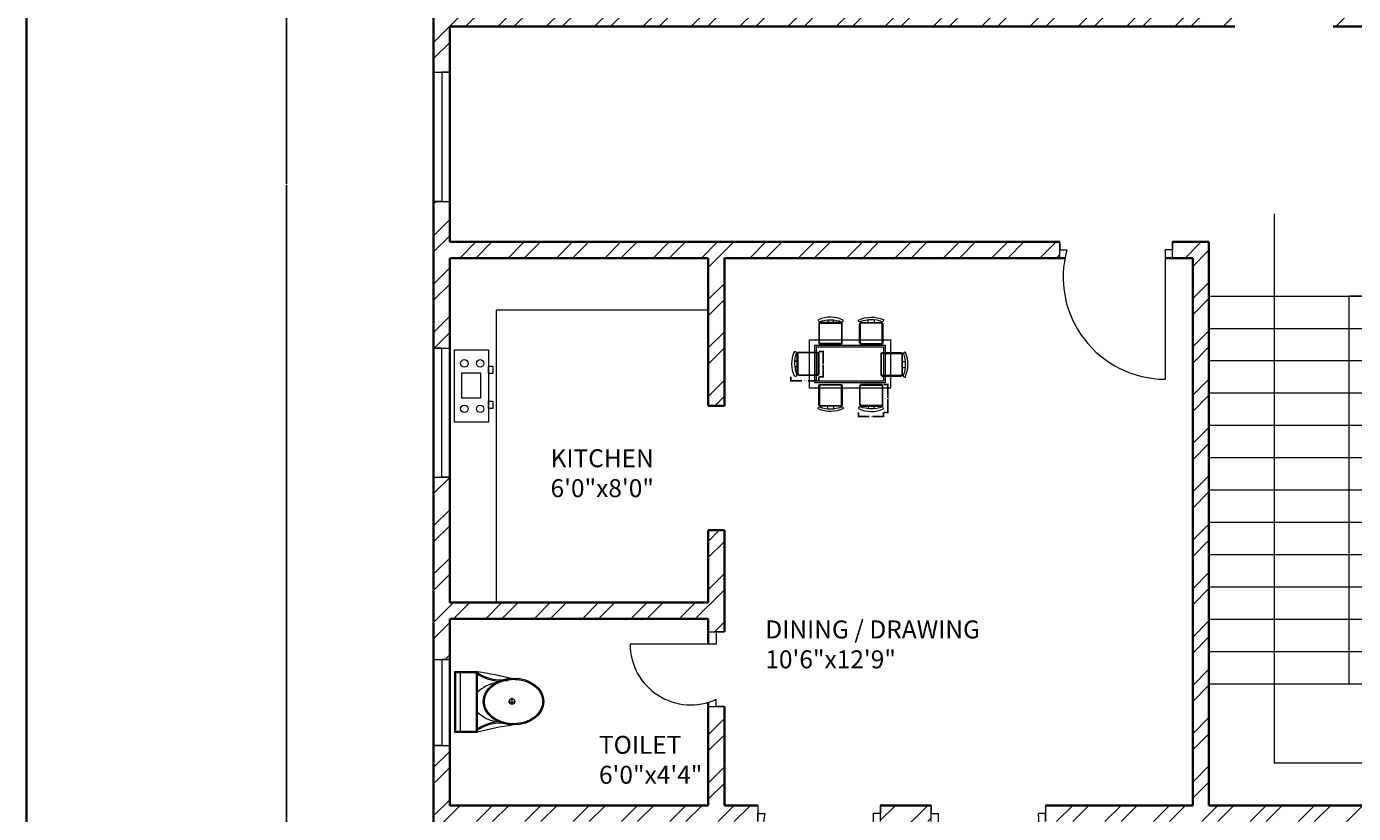
# Model space of a CAD drawing. Units: inches. Extents: x 1944 to 3454, y 1352 to 3055.
# Tile 2 of 17: x 1944 to 2314, y 1681 to 1900. Entities that reach past the tile are written whole.
import ezdxf

# ---------------------------------------------------------------- set-up
doc = ezdxf.new("R2010")
doc.units = ezdxf.units.IN
for name, color, linetype, lineweight in [('A-ANNO-DIMS', 2, 'Continuous', 18), ('A-ANNO-TTLB', 7, 'Continuous', 35), ('A-AREA-IDEN', 7, 'Continuous', 18), ('A-DOOR', 3, 'Continuous', 20), ('A-EQPM', 9, 'Continuous', 18), ('A-FLOR-CASE', 8, 'Continuous', 20), ('A-FLOR-FIXT', 9, 'Continuous', 18), ('A-FLOR-STRS', 7, 'Continuous', 20), ('A-FURN', 8, 'Continuous', 13), ('A-GLAZ', 4, 'Continuous', 18), ('A-WALL', 7, 'Continuous', 35), ('A-WALL-PATT', 252, 'Continuous', 13)]:
    doc.layers.add(name, color=color, linetype=linetype, lineweight=lineweight)
doc.styles.get("Standard").update_dxf_attribs({"font": 'arial.ttf'})
doc.dimstyles.get("Standard").update_dxf_attribs({"dimtxt": 0.18, "dimasz": 0.18, "dimexe": 0.18, "dimexo": 0.0625, "dimgap": 0.09, "dimtad": 0, "dimtih": 1, "dimtoh": 1, "dimdec": 4, "dimzin": 0, "dimdsep": 46, "dimtxsty": 'Standard', "dimcen": 0.09, "dimadec": 0, "dimazin": 0, "dimtfac": 1, "dimtdec": 4, "dimtofl": 0, "dimtmove": 0, "dimatfit": 3, "dimfxl": 1, "dimtolj": 1, "dimtzin": 0, "dimarcsym": 0})

# ---------------------------------------------------------------- blocks, each defined once
blk = doc.blocks.new('A$C31115884')
for p, q in [((283, 498), (223, 498)), ((258, 466), (258, 523)), ((0, 200), (0, 0)), ((520, 200), (0, 200)), ((10, 190), (10, 10)), ((510, 190), (10, 190)), ((510, 10), (510, 190)), ((520, 0), (520, 200)), ((510, 54), (0, 54)), ((10, 10), (510, 10)), ((0, 0), (520, 0))]:
    blk.add_line(p, q)
blk.add_circle((256, 496), 23.6)
for centre, radius, start, end in [((2778, -205), 2807, 165.4549, 171.7133), ((-295, 403), 365, 324.2091, 9.3499), ((-295, 403), 375, 324.2091, 9.3499), ((806, 403), 365, 170.6501, 215.7909), ((3237, 905), 2807, 188.2867, 194.5451), ((384, 406), 293, 190.2774, 224.1564), ((139, 406), 293, 315.8436, 2.6563), ((806, 403), 375, 179.2036, 215.7909)]:
    blk.add_arc(centre, radius, start, end)
blk.add_ellipse((256, 510), major_axis=(0, -261), ratio=0.772727)
blk.add_open_spline([(256, 259), (263, 259), (270, 260), (288, 262), (299, 265), (320, 273), (330, 278), (350, 291), (360, 299), (378, 316), (386, 326), (402, 347), (409, 358), (421, 383), (427, 395), (436, 422), (440, 436), (445, 465), (447, 480), (448, 509), (448, 524), (445, 553), (443, 568), (436, 596), (432, 610), (422, 636), (416, 649), (402, 672), (395, 683), (379, 703), (370, 712), (351, 728), (341, 735), (321, 746), (310, 751), (289, 757), (278, 759), (256, 761), (245, 761), (223, 757), (212, 754), (191, 746), (181, 741), (161, 728), (151, 720), (133, 703), (125, 693), (110, 672), (103, 660), (90, 636), (85, 623), (76, 596), (72, 582), (67, 553), (66, 538), (64, 509), (65, 494), (68, 465), (70, 450), (77, 422), (81, 408), (91, 382), (97, 370), (111, 346), (118, 335), (135, 316), (144, 307), (162, 291), (172, 284), (193, 273), (203, 269), (225, 262), (236, 260), (250, 259), (253, 259), (256, 259)], degree=3, knots=[0, 0, 0, 0, 0.110105, 0.110105, 0.285049, 0.285049, 0.459994, 0.459994, 0.634938, 0.634938, 0.809882, 0.809882, 0.984827, 0.984827, 1.159771, 1.159771, 1.334715, 1.334715, 1.50966, 1.50966, 1.684604, 1.684604, 1.859549, 1.859549, 2.034493, 2.034493, 2.209437, 2.209437, 2.384382, 2.384382, 2.559326, 2.559326, 2.73427, 2.73427, 2.909215, 2.909215, 3.084159, 3.084159, 3.259103, 3.259103, 3.434048, 3.434048, 3.608992, 3.608992, 3.783936, 3.783936, 3.958881, 3.958881, 4.133825, 4.133825, 4.30877, 4.30877, 4.483714, 4.483714, 4.658658, 4.658658, 4.833603, 4.833603, 5.008547, 5.008547, 5.183491, 5.183491, 5.358436, 5.358436, 5.53338, 5.53338, 5.708324, 5.708324, 5.883269, 5.883269, 6.058213, 6.058213, 6.233158, 6.233158, 6.283185, 6.283185, 6.283185, 6.283185])
blk = doc.blocks.new('COOKTOP-4B-01')
for points in [[(0, 20.18), (9.48, 20.18), (9.48, 0), (0, 0)], [(9.48, 15.59), (10.71, 15.59), (10.71, 13.59), (9.48, 13.59)], [(2, 13.79), (7.26, 13.79), (7.26, 6.73), (2, 6.73)], [(9.48, 5.81), (10.71, 5.81), (10.71, 3.8), (9.48, 3.8)]]:
    blk.add_lwpolyline(points, close=True)
for centre in [(2.74, 16.38), (7.14, 16.38), (2.74, 3.71), (7.14, 3.71)]:
    blk.add_circle(centre, 1.05)
blk = doc.blocks.new('DOOR-SWING-24IN-08')
for p, q in [((21.75, 20.75), (26.25, 20.75)), ((26.25, 20.75), (24, 20.75)), ((24, 20.75), (24, 19.34)), ((24, 19.34), (24, 17.34)), ((24, 17.34), (0, 17.34)), ((21.75, 0), (26.25, 0)), ((24, 0), (24, 2)), ((26.25, 0), (24, 0))]:
    blk.add_line(p, q)
blk.add_arc((16.9, 17.34), 16.9, 180, 294.8206)
blk = doc.blocks.new('DOOR-SWING-36IN-07')
for p, q in [((0, 38.25), (0, 33.75)), ((34.17, 33.75), (34.17, 38.25)), ((34.17, 38.25), (34.17, 36)), ((0, 33.75), (0, 36)), ((0, 36), (2, 36)), ((34.17, 36), (32.17, 36)), ((32.17, 36), (32.17, 0))]:
    blk.add_line(p, q)
blk.add_arc((32.17, 30.64), 30.64, 169.9223, 270)
blk = doc.blocks.new('DOOR-SWING-36IN-08')
for p, q in [((0, 33.75), (0, 38.25)), ((0, 38.25), (0, 38.25)), ((0, 38.25), (0, 36)), ((31.9, 38.25), (31.9, 33.75)), ((0, 36), (2, 36)), ((2, 36), (2, 0)), ((31.9, 36), (29.9, 36)), ((31.9, 33.75), (31.9, 36))]:
    blk.add_line(p, q)
blk.add_arc((-3.46, 33.05), 33.5, 279.3869, 5.0549)
blk = doc.blocks.new('DOOR-SWING-36IN-11')
for p, q in [((0, 33.75), (0, 38.25)), ((0, 38.25), (0, 36)), ((31.41, 33.75), (31.41, 38.25)), ((31.41, 38.25), (31.41, 36)), ((0, 36), (2, 36)), ((31.41, 36), (29.41, 36)), ((29.41, 36), (29.41, 0))]:
    blk.add_line(p, q)
blk.add_arc((29.41, 28.43), 28.43, 164.5673, 270)
blk = doc.blocks.new('WINDOW-PLAN-36.00IN-01')
for p, q in [((0, 36), (4.5, 36)), ((4.5, 36), (2.25, 36)), ((2.25, 36), (2.25, 0)), ((2.25, 0), (0, 0)), ((0, 0), (4.5, 0))]:
    blk.add_line(p, q)
blk = doc.blocks.new('WINDOW-PLAN-24.00IN-01')
for p, q in [((2.25, 24), (0, 24)), ((0, 24), (4.5, 24)), ((2.25, 0), (2.25, 24)), ((0, 0), (4.5, 0)), ((4.5, 0), (2.25, 0))]:
    blk.add_line(p, q)
blk = doc.blocks.new('STAIR-TWO-FLIGHT-01')
for p, q in [((18.12, 152.99), (18.12, 0)), ((0, 130.08), (78, 130.08)), ((78, 130.08), (39, 130.08)), ((39, 130.08), (39, 22.08)), ((0, 121.08), (78, 121.08)), ((0, 112.08), (78, 112.08)), ((0, 103.08), (78, 103.08)), ((0, 94.08), (78, 94.08)), ((0, 85.08), (78, 85.08)), ((0, 76.08), (78, 76.08)), ((0, 67.08), (78, 67.08)), ((61.93, 0), (61.93, 67.08)), ((0, 58.08), (78, 58.08)), ((0, 49.08), (78, 49.08)), ((0, 40.08), (78, 40.08)), ((0, 31.08), (78, 31.08)), ((0, 22.08), (78, 22.08)), ((18.12, 0), (61.93, 0))]:
    blk.add_line(p, q)
blk = doc.blocks.new('TABLE-DINING-01')
for points in [[(0, 13.51), (22.52, 13.51), (22.52, 0), (0, 0)], [(0, 13.51), (22.52, 13.51), (22.52, 0), (0, 0)], [(1.5, 12.01), (21.02, 12.01), (21.02, 1.5), (1.5, 1.5)], [(1.5, 12.01), (21.02, 12.01), (21.02, 1.5), (1.5, 1.5)], [(1.95, 11.56), (20.57, 11.56), (20.57, 1.95), (1.95, 1.95)], [(1.95, 11.56), (20.57, 11.56), (20.57, 1.95), (1.95, 1.95)]]:
    blk.add_lwpolyline(points, close=True)
blk = doc.blocks.new('CHAIR-DINING-01')
for points in [[(0.48, 6.23, -0.578392), (0.02, 6.74, -0.214524), (6.94, 6.84, -0.552014), (6.62, 6.28, 0.175809), (0.48, 6.23)], [(6.44, 6.03, -0.414214), (6.84, 5.63), (6.84, 0.4, -0.414214), (6.44, 0), (0.74, 0, -0.414214), (0.34, 0.4), (0.34, 5.63, -0.414214), (0.74, 6.03), (6.44, 6.03)], [(2.74, 6.03), (2.74, 6.75, 0.064759)]]:
    blk.add_lwpolyline(points, format="xyb")
blk.add_lwpolyline([(6.44, 5.85), (0.92, 5.85, 0.414214), (0.52, 5.45), (0.52, 0.58, 0.414214), (0.92, 0.18), (6.44, 0.18, 0.512069), (6.66, 0.58), (6.66, 5.45, 0.512069)], format="xyb", close=True)
blk.add_lwpolyline([(4.34, 6.77), (4.34, 6.03)])
blk = doc.blocks.new('CHAIR-DINING-07')
for points in [[(1.3, 0.48, -0.578392), (0.79, 0.02, -0.214524), (0.7, 6.94, -0.552014), (1.25, 6.62, 0.175809), (1.3, 0.48)], [(1.5, 6.44, -0.414214), (1.9, 6.84), (7.13, 6.84, -0.414214), (7.53, 6.44), (7.53, 0.74, -0.414214), (7.13, 0.34), (1.9, 0.34, -0.414214), (1.5, 0.74), (1.5, 6.44)], [(1.5, 2.74), (0.78, 2.74, 0.064759)]]:
    blk.add_lwpolyline(points, format="xyb")
blk.add_lwpolyline([(0.77, 4.34), (1.5, 4.34)])
blk.add_lwpolyline([(1.68, 6.44), (1.68, 0.92, 0.414214), (2.08, 0.52), (6.95, 0.52, 0.414214), (7.35, 0.92), (7.35, 6.44, 0.512069), (6.95, 6.66), (2.08, 6.66, 0.512069)], format="xyb", close=True)
blk = doc.blocks.new('CHAIR-DINING-09')
for points in [[(6.24, 1.5), (0.55, 1.5, -0.414214), (0.15, 1.9), (0.15, 7.13, -0.414214), (0.55, 7.53), (6.24, 7.53, -0.414214), (6.64, 7.13), (6.64, 1.9, -0.414214), (6.24, 1.5)], [(6.5, 1.3, -0.578392), (6.97, 0.79, -0.214524), (0.04, 0.7, -0.552014), (0.37, 1.25, 0.175809), (6.5, 1.3)], [(4.24, 1.5), (4.24, 0.78, 0.064759)]]:
    blk.add_lwpolyline(points, format="xyb")
blk.add_lwpolyline([(0.55, 1.68), (6.06, 1.68, 0.414214), (6.46, 2.08), (6.46, 6.95, 0.414214), (6.06, 7.35), (0.55, 7.35, 0.512069), (0.33, 6.95), (0.33, 2.08, 0.512069)], format="xyb", close=True)
blk.add_lwpolyline([(2.65, 0.77), (2.65, 1.5)])
blk = doc.blocks.new('CHAIR-DINING-10')
for points in [[(6.44, 1.5, 0.414214), (6.84, 1.9), (6.84, 7.13, 0.414214), (6.44, 7.53), (0.74, 7.53, 0.414214), (0.34, 7.13), (0.34, 1.9, 0.414214), (0.74, 1.5), (6.44, 1.5)], [(6.62, 1.25, -0.175809), (0.48, 1.3, 0.578392), (0.02, 0.79, 0.214524), (6.94, 0.7, 0.552014), (6.62, 1.25, -0.065079)], [(2.74, 1.5), (2.74, 0.78, -0.064759)]]:
    blk.add_lwpolyline(points, format="xyb")
blk.add_lwpolyline([(6.44, 1.68), (0.92, 1.68, -0.414214), (0.52, 2.08), (0.52, 6.95, -0.414214), (0.92, 7.35), (6.44, 7.35, -0.512069), (6.66, 6.95), (6.66, 2.08, -0.512069)], format="xyb", close=True)
blk.add_lwpolyline([(4.34, 0.77), (4.34, 1.5)])
blk = doc.blocks.new('CHAIR-DINING-11')
for points in [[(6.44, 1.5, 0.414214), (6.84, 1.9), (6.84, 7.13, 0.414214), (6.44, 7.53), (0.74, 7.53, 0.414214), (0.34, 7.13), (0.34, 1.9, 0.414214), (0.74, 1.5), (6.44, 1.5)], [(6.62, 1.25, -0.175809), (0.48, 1.3, 0.578392), (0.02, 0.79, 0.214524), (6.94, 0.7, 0.552014), (6.62, 1.25, -0.065079)], [(2.74, 1.5), (2.74, 0.78, -0.064759)]]:
    blk.add_lwpolyline(points, format="xyb")
blk.add_lwpolyline([(6.44, 1.68), (0.92, 1.68, -0.414214), (0.52, 2.08), (0.52, 6.95, -0.414214), (0.92, 7.35), (6.44, 7.35, -0.512069), (6.66, 6.95), (6.66, 2.08, -0.512069)], format="xyb", close=True)
blk.add_lwpolyline([(4.34, 0.77), (4.34, 1.5)])
blk = doc.blocks.new('*D152')
at = {"layer": 'A-ANNO-DIMS', "color": 0, "lineweight": -2, "transparency": 16777216}
for p, q in [((2156.87, 1802.48), (2156.87, 1801.2)), ((2157.05, 1801.38), (2159.88, 1801.38)), ((2164.48, 1801.38), (2161.65, 1801.38)), ((2164.66, 1802.48), (2164.66, 1801.2))]:
    blk.add_line(p, q, dxfattribs=at)
at = {"layer": 'A-ANNO-DIMS', "color": 0, "transparency": 16777216}
for points in [[(2157.05, 1801.41), (2157.05, 1801.35), (2156.87, 1801.38)], [(2164.48, 1801.41), (2164.48, 1801.35), (2164.66, 1801.38)]]:
    blk.add_solid(points, dxfattribs=at)
at = {"layer": 'Defpoints', "color": 0, "transparency": 16777216}
for p in [(2156.87, 1802.54), (2164.66, 1802.54), (2164.66, 1801.38)]:
    blk.add_point(p, dxfattribs=at)
at = {"layer": 'A-ANNO-DIMS', "color": 0, "transparency": 16777216, "insert": (2160.76, 1801.38), "char_height": 0.18, "attachment_point": 5}
blk.add_mtext('\\A1;CHAIR 8 TYP.', dxfattribs=at)
blk = doc.blocks.new('*D153')
at = {"layer": 'A-ANNO-DIMS', "color": 0, "lineweight": -2, "transparency": 16777216}
for p, q in [((2164.73, 1809.57), (2166.01, 1809.57)), ((2165.83, 1809.39), (2165.83, 1806.24)), ((2165.83, 1802.72), (2165.83, 1805.88)), ((2164.73, 1802.54), (2166.01, 1802.54))]:
    blk.add_line(p, q, dxfattribs=at)
at = {"layer": 'A-ANNO-DIMS', "color": 0, "transparency": 16777216}
for points in [[(2165.8, 1809.39), (2165.86, 1809.39), (2165.83, 1809.57)], [(2165.8, 1802.72), (2165.86, 1802.72), (2165.83, 1802.54)]]:
    blk.add_solid(points, dxfattribs=at)
at = {"layer": 'Defpoints', "color": 0, "transparency": 16777216}
for p in [(2164.66, 1809.57), (2165.83, 1809.57), (2164.66, 1802.54)]:
    blk.add_point(p, dxfattribs=at)
at = {"layer": 'A-ANNO-DIMS', "color": 0, "transparency": 16777216, "insert": (2165.83, 1806.06), "char_height": 0.18, "attachment_point": 5}
blk.add_mtext('\\A1;7 TYP.', dxfattribs=at)
blk = doc.blocks.new('*D158')
at = {"layer": 'A-ANNO-DIMS', "color": 0, "lineweight": -2, "transparency": 16777216}
for p, q in [((2182.73, 1800.38), (2184.02, 1800.38)), ((2183.84, 1800.2), (2183.84, 1796.66)), ((2183.84, 1792.76), (2183.84, 1796.3)), ((2182.73, 1792.58), (2184.02, 1792.58))]:
    blk.add_line(p, q, dxfattribs=at)
at = {"layer": 'A-ANNO-DIMS', "color": 0, "transparency": 16777216}
for points in [[(2183.81, 1800.2), (2183.87, 1800.2), (2183.84, 1800.38)], [(2183.81, 1792.76), (2183.87, 1792.76), (2183.84, 1792.58)]]:
    blk.add_solid(points, dxfattribs=at)
at = {"layer": 'Defpoints', "color": 0, "transparency": 16777216}
for p in [(2182.67, 1800.38), (2183.84, 1800.38), (2182.67, 1792.58)]:
    blk.add_point(p, dxfattribs=at)
at = {"layer": 'A-ANNO-DIMS', "color": 0, "transparency": 16777216, "insert": (2183.84, 1796.48), "char_height": 0.18, "attachment_point": 5}
blk.add_mtext('\\A1;CHAIR 8 TYP.', dxfattribs=at)
blk = doc.blocks.new('*D159')
at = {"layer": 'A-ANNO-DIMS', "color": 0, "lineweight": -2, "transparency": 16777216}
for p, q in [((2175.64, 1792.52), (2175.64, 1791.23)), ((2175.82, 1791.41), (2178.69, 1791.41)), ((2182.49, 1791.41), (2179.61, 1791.41)), ((2182.67, 1792.52), (2182.67, 1791.23))]:
    blk.add_line(p, q, dxfattribs=at)
at = {"layer": 'A-ANNO-DIMS', "color": 0, "transparency": 16777216}
for points in [[(2175.82, 1791.44), (2175.82, 1791.38), (2175.64, 1791.41)], [(2182.49, 1791.44), (2182.49, 1791.38), (2182.67, 1791.41)]]:
    blk.add_solid(points, dxfattribs=at)
at = {"layer": 'Defpoints', "color": 0, "transparency": 16777216}
for p in [(2175.64, 1792.58), (2182.67, 1792.58), (2182.67, 1791.41)]:
    blk.add_point(p, dxfattribs=at)
at = {"layer": 'A-ANNO-DIMS', "color": 0, "transparency": 16777216, "insert": (2179.15, 1791.41), "char_height": 0.18, "attachment_point": 5}
blk.add_mtext('\\A1;7 TYP.', dxfattribs=at)
blk = doc.blocks.new('*D185')
at = {"layer": 'A-ANNO-DIMS', "color": 0, "lineweight": -2, "transparency": 16777216}
for p, q in [((2122.1, 2222.6), (2016.19, 2222.6)), ((2016.37, 2222.42), (2016.37, 1856.28)), ((2016.37, 1489.78), (2016.37, 1855.91)), ((2123.11, 1489.6), (2016.19, 1489.6))]:
    blk.add_line(p, q, dxfattribs=at)
at = {"layer": 'A-ANNO-DIMS', "color": 0, "transparency": 16777216}
for points in [[(2016.34, 2222.42), (2016.4, 2222.42), (2016.37, 2222.6)], [(2016.34, 1489.78), (2016.4, 1489.78), (2016.37, 1489.6)]]:
    blk.add_solid(points, dxfattribs=at)
at = {"layer": 'Defpoints', "color": 0, "transparency": 16777216}
for p in [(2016.37, 2222.6), (2122.17, 2222.6), (2123.17, 1489.6)]:
    blk.add_point(p, dxfattribs=at)
at = {"layer": 'A-ANNO-DIMS', "color": 0, "transparency": 16777216, "insert": (2016.37, 1856.1), "char_height": 0.18, "attachment_point": 5}
blk.add_mtext('\\A1;733', dxfattribs=at)

msp = doc.modelspace()

# ---------------------------------------------------------------- hatches: boundary and pattern name
at = {"layer": 'A-WALL-PATT'}
h = msp.add_hatch(dxfattribs=at)
h.set_pattern_fill('ANSI32', color=256)
h.paths.add_polyline_path([(2061.822, 2177.596), (2158.181, 2177.596), (2158.181, 2179.846), (2158.181, 2182.096), (2057.322, 2182.096), (2057.322, 2123.452), (2061.822, 2123.452)])
h.paths.add_polyline_path([(2258.993, 2179.846), (2258.993, 2182.096), (2218.838, 2182.096), (2218.838, 2177.596), (2258.993, 2177.596)])
h.paths.add_polyline_path([(2315.822, 2177.596), (2322.722, 2177.596), (2322.722, 2182.096), (2303.186, 2182.096), (2303.186, 2177.596), (2311.322, 2177.596), (2311.322, 2033.596), (2231.355, 2033.596), (2231.355, 2029.096), (2311.322, 2029.096), (2311.322, 1904.596), (2307.941, 1904.596), (2307.941, 1900.096), (2319.277, 1900.096), (2319.277, 1902.346), (2319.277, 1904.596), (2315.822, 1904.596), (2315.822, 2029.096), (2394.855, 2029.096), (2394.855, 2033.596), (2315.822, 2033.596)])
h.paths.add_polyline_path([(2407.334, 2182.096), (2366.1, 2182.096), (2366.1, 2177.596), (2407.334, 2177.596), (2407.334, 2179.846)])
h.paths.add_polyline_path([(2440.322, 2177.596), (2443.866, 2177.596), (2443.866, 2182.096), (2431.827, 2182.096), (2431.827, 2179.846), (2431.827, 2177.596), (2435.822, 2177.596), (2435.822, 2033.596), (2430.464, 2033.596), (2430.464, 2029.096), (2445.372, 2029.096), (2445.372, 2031.346), (2445.372, 2033.596), (2440.322, 2033.596)])
h.paths.add_polyline_path([(2569.822, 2182.096), (2466.481, 2182.096), (2466.481, 2177.596), (2565.322, 2177.596), (2565.322, 2123.452), (2569.822, 2123.452)])
h.paths.add_polyline_path([(2569.822, 2063.452), (2567.572, 2063.452), (2565.322, 2063.452), (2565.322, 2033.596), (2478.08, 2033.596), (2476.822, 2033.596), (2476.822, 2028.698), (2476.822, 2020.069), (2481.322, 2020.069), (2481.322, 2029.096), (2565.322, 2029.096), (2565.322, 2014.5), (2569.822, 2014.5)])
h.paths.add_polyline_path([(2569.822, 1978.5), (2565.322, 1978.5), (2565.322, 1957.096), (2481.322, 1957.096), (2481.322, 1990.369), (2476.822, 1990.369), (2476.822, 1957.096), (2476.822, 1952.596), (2476.822, 1947.471), (2481.322, 1947.471), (2481.322, 1952.596), (2565.322, 1952.596), (2565.322, 1943.2), (2569.822, 1943.2)])
h.paths.add_polyline_path([(2569.822, 1919.2), (2565.322, 1919.2), (2565.322, 1904.596), (2481.322, 1904.596), (2481.322, 1928.596), (2476.822, 1928.596), (2476.822, 1904.596), (2350.518, 1904.596), (2350.518, 1900.096), (2476.822, 1900.096), (2565.322, 1900.096), (2565.322, 1895.596), (2565.322, 1887.047), (2569.822, 1887.047)])
h.paths.add_polyline_path([(2280.492, 1904.596), (2150.322, 1904.596), (2150.322, 1926.68), (2148.072, 1926.68), (2145.822, 1926.68), (2145.822, 1904.596), (2061.822, 1904.596), (2061.822, 1914.977), (2059.572, 1914.977), (2057.322, 1914.977), (2057.322, 1887.362), (2061.822, 1887.362), (2061.822, 1900.096), (2150.322, 1900.096), (2280.492, 1900.096), (2280.492, 1902.346)])
h.paths.add_polyline_path([(2150.322, 1957.096), (2150.322, 1986.22), (2145.822, 1986.22), (2145.822, 1957.096), (2061.822, 1957.096), (2061.822, 1975.678), (2057.322, 1975.678), (2057.322, 1938.977), (2061.822, 1938.977), (2061.822, 1952.596), (2145.822, 1952.596), (2145.822, 1947.985), (2150.322, 1947.985), (2150.322, 1952.596)])
h.paths.add_polyline_path([(2061.822, 2063.452), (2057.322, 2063.452), (2057.322, 2011.678), (2061.822, 2011.678), (2061.822, 2029.096), (2145.288, 2029.096), (2145.822, 2029.096), (2145.822, 2019.118), (2150.322, 2019.118), (2150.322, 2029.096), (2150.322, 2033.596), (2147.022, 2033.596), (2061.822, 2033.596)])
h.paths.add_polyline_path([(2061.822, 1835.596), (2133.822, 1835.596), (2133.822, 1794.415), (2138.322, 1794.415), (2138.322, 1835.596), (2231.726, 1835.596), (2231.726, 1840.096), (2061.822, 1840.096), (2061.822, 1851.362), (2057.322, 1851.362), (2057.322, 1810.528), (2061.822, 1810.528)])
h.paths.add_polyline_path([(2061.822, 1774.528), (2059.572, 1774.528), (2057.322, 1774.528), (2057.322, 1723.746), (2061.822, 1723.746), (2061.822, 1735.096), (2133.822, 1735.096), (2133.822, 1731.415), (2138.322, 1731.415), (2138.322, 1759.737), (2133.822, 1759.737), (2133.822, 1739.596), (2061.822, 1739.596)])
h.paths.add_polyline_path([(2061.822, 1678.596), (2147.597, 1678.596), (2147.597, 1680.846), (2147.597, 1683.096), (2138.322, 1683.096), (2138.322, 1710.66), (2136.072, 1710.66), (2133.822, 1710.66), (2133.822, 1683.096), (2061.822, 1683.096), (2061.822, 1699.746), (2057.322, 1699.746), (2057.322, 1645.751), (2061.822, 1645.751)])
h.paths.add_polyline_path([(2061.822, 1585.751), (2057.322, 1585.751), (2057.322, 1530.096), (2158.703, 1530.096), (2158.703, 1534.596), (2061.822, 1534.596)])
h.paths.add_polyline_path([(2191.322, 1678.596), (2195.889, 1678.596), (2195.889, 1683.096), (2181.763, 1683.096), (2181.763, 1680.846), (2181.763, 1678.596), (2186.822, 1678.596), (2186.822, 1534.596), (2181.354, 1534.596), (2181.354, 1530.096), (2196.54, 1530.096), (2196.54, 1532.346), (2196.54, 1534.596), (2191.322, 1534.596)])
h.paths.add_polyline_path([(2315.822, 1678.596), (2402.014, 1678.596), (2402.014, 1683.096), (2355.822, 1683.096), (2355.822, 1835.596), (2360.838, 1835.596), (2360.838, 1840.096), (2351.322, 1840.096), (2351.322, 1683.096), (2273.322, 1683.096), (2273.322, 1840.096), (2263.134, 1840.096), (2263.134, 1837.846), (2263.134, 1835.596), (2268.822, 1835.596), (2268.822, 1683.096), (2227.793, 1683.096), (2227.793, 1678.596), (2311.322, 1678.596), (2311.322, 1534.596), (2302.384, 1534.596), (2302.384, 1530.096), (2324.521, 1530.096), (2324.521, 1532.346), (2324.521, 1534.596), (2315.822, 1534.596)])
h.paths.add_polyline_path([(2440.322, 1678.596), (2443.656, 1678.596), (2443.656, 1683.096), (2432.614, 1683.096), (2432.614, 1680.846), (2432.614, 1678.596), (2435.822, 1678.596), (2435.822, 1534.596), (2440.322, 1534.596)])
h.paths.add_polyline_path([(2409.913, 1534.596), (2369.033, 1534.596), (2369.033, 1530.096), (2409.913, 1530.096)])
h.paths.add_polyline_path([(2259.529, 1532.346), (2259.529, 1534.596), (2218.889, 1534.596), (2218.889, 1532.346), (2218.889, 1530.096), (2259.529, 1530.096)])
h.paths.add_polyline_path([(2569.822, 1584.389), (2567.572, 1584.389), (2565.322, 1584.389), (2565.322, 1534.596), (2465.892, 1534.596), (2465.892, 1530.096), (2569.822, 1530.096)])
h.paths.add_polyline_path([(2505.567, 1530.096), (2501.067, 1530.096), (2501.067, 1494.096), (2381.067, 1494.096), (2381.067, 1530.096), (2376.567, 1530.096), (2376.567, 1489.596), (2381.067, 1489.596), (2505.567, 1489.596), (2505.567, 1494.096)])
h.paths.add_polyline_path([(2127.673, 1530.096), (2123.173, 1530.096), (2123.173, 1489.596), (2127.673, 1489.596), (2252.173, 1489.596), (2252.173, 1494.096), (2252.173, 1530.096), (2247.673, 1530.096), (2247.673, 1494.096), (2127.673, 1494.096)])
h.paths.add_polyline_path([(2251.167, 2222.596), (2126.667, 2222.596), (2122.167, 2222.596), (2122.167, 2182.096), (2126.667, 2182.096), (2126.667, 2218.096), (2210.667, 2218.096), (2234.667, 2218.096), (2246.667, 2218.096), (2246.667, 2182.096), (2251.167, 2182.096), (2251.167, 2218.096)])
h.paths.add_polyline_path([(2501.916, 2222.596), (2497.416, 2222.596), (2372.916, 2222.596), (2372.916, 2218.096), (2372.916, 2182.096), (2377.416, 2182.096), (2377.416, 2218.096), (2497.416, 2218.096), (2497.416, 2182.096), (2501.916, 2182.096)])
h.paths.add_polyline_path([(2569.822, 1700.442), (2565.322, 1700.442), (2565.322, 1683.096), (2493.322, 1683.096), (2493.322, 1709.096), (2488.822, 1709.096), (2488.822, 1683.096), (2475.416, 1683.096), (2475.416, 1680.846), (2475.416, 1678.596), (2488.822, 1678.596), (2565.322, 1678.596), (2565.322, 1644.389), (2569.822, 1644.389)])
h.paths.add_polyline_path([(2569.822, 1773.506), (2565.322, 1773.506), (2565.322, 1739.596), (2493.322, 1739.596), (2493.322, 1754.002), (2488.822, 1754.002), (2488.822, 1729.846), (2491.072, 1729.846), (2493.322, 1729.846), (2493.322, 1735.096), (2565.322, 1735.096), (2565.322, 1724.442), (2569.822, 1724.442)])
h.paths.add_polyline_path([(2569.822, 1851.047), (2567.572, 1851.047), (2565.322, 1851.047), (2565.322, 1840.096), (2395.039, 1840.096), (2395.039, 1837.846), (2395.039, 1835.596), (2488.822, 1835.596), (2488.822, 1798.423), (2493.322, 1798.423), (2493.322, 1835.596), (2565.322, 1835.596), (2565.322, 1809.506), (2569.822, 1809.506)])
h.paths.add_polyline_path([(2347.275, 1955.576), (2414.024, 1955.576), (2414.024, 1974.234), (2347.275, 1974.234)], flags=9)
h.paths.add_polyline_path([(2509.756, 1990.497), (2542.915, 1990.497), (2542.915, 2009.154), (2509.756, 2009.154)], flags=9)

# ---------------------------------------------------------------- linework, layer by layer
at = {"layer": 'A-ANNO-TTLB'}
msp.add_lwpolyline([(1943.914, 3054.605), (3453.633, 3054.605), (3453.633, 1351.76), (1943.914, 1351.76)], close=True, dxfattribs=at)
at = {"layer": 'A-FLOR-CASE'}
for p, q in [((2133.822, 1821.056), (2074.701, 1821.056)), ((2074.701, 1821.056), (2074.701, 1739.596))]:
    msp.add_line(p, q, dxfattribs=at)
at = {"layer": 'A-FURN'}
for points in [[(2164.848, 1817.865, -0.1758092), (2170.982, 1817.819, 0.5783921), (2171.447, 1818.33, 0.2145244), (2164.523, 1818.423, 0.552014), (2164.848, 1817.865, -0.065079)], [(2164.848, 1817.865, -0.1758092), (2170.982, 1817.819, 0.5783921), (2171.447, 1818.33, 0.2145244), (2164.523, 1818.423, 0.552014), (2164.848, 1817.865, -0.065079)], [(2170.722, 1817.619), (2165.027, 1817.619, 0.4142136), (2164.629, 1817.221), (2164.629, 1811.985, 0.4142136), (2165.027, 1811.586), (2170.722, 1811.586, 0.4142136), (2171.12, 1811.985), (2171.12, 1817.221, 0.4142136), (2170.722, 1817.619)], [(2170.722, 1817.619), (2165.027, 1817.619, 0.4142136), (2164.629, 1817.221), (2164.629, 1811.985, 0.4142136), (2165.027, 1811.586), (2170.722, 1811.586, 0.4142136), (2171.12, 1811.985), (2171.12, 1817.221, 0.4142136), (2170.722, 1817.619)], [(2168.722, 1817.619), (2168.722, 1818.339, -0.0647586)], [(2168.722, 1817.619), (2168.722, 1818.339, -0.0647586)], [(2158.431, 1803.053, -0.5783921), (2157.92, 1802.588, -0.2145244), (2157.827, 1809.512, -0.552014), (2158.384, 1809.187, 0.1758094), (2158.431, 1803.053)], [(2158.631, 1809.007, -0.4142136), (2159.029, 1809.406), (2164.265, 1809.406, -0.4142136), (2164.663, 1809.007), (2164.663, 1803.313, -0.4142136), (2164.265, 1802.915), (2159.029, 1802.915, -0.4142136), (2158.631, 1803.313), (2158.631, 1809.007)], [(2187.954, 1808.813, 0.4142136), (2187.556, 1809.211), (2182.32, 1809.211, 0.4142136), (2181.922, 1808.813), (2181.922, 1803.118, 0.4142136), (2182.32, 1802.72), (2187.556, 1802.72, 0.4142136), (2187.954, 1803.118), (2187.954, 1808.813)], [(2187.954, 1808.812, 0.4142136), (2187.556, 1809.211), (2182.32, 1809.211, 0.4142136), (2181.922, 1808.812), (2181.922, 1803.118, 0.4142136), (2182.32, 1802.72), (2187.556, 1802.72, 0.4142136), (2187.954, 1803.118), (2187.954, 1808.812)], [(2188.201, 1808.992, -0.1758092), (2188.154, 1802.858, 0.5783921), (2188.665, 1802.393, 0.2145244), (2188.758, 1809.317, 0.552014), (2188.201, 1808.992, -0.065079)], [(2188.201, 1808.992, -0.1758092), (2188.154, 1802.858, 0.5783921), (2188.665, 1802.393, 0.2145244), (2188.758, 1809.317, 0.552014), (2188.201, 1808.992, -0.065079)], [(2158.631, 1805.313), (2157.91, 1805.313, 0.0647586)], [(2187.954, 1805.118), (2188.675, 1805.118, -0.0647586)], [(2187.954, 1805.118), (2188.675, 1805.118, -0.0647586)]]:
    msp.add_lwpolyline(points, format="xyb", dxfattribs=at)
for points in [[(2165.03, 1817.44), (2170.542, 1817.44, -0.4142136), (2170.941, 1817.041), (2170.941, 1812.164, -0.4142136), (2170.542, 1811.766), (2165.03, 1811.766, -0.5120695), (2164.808, 1812.164), (2164.808, 1817.041, -0.5120695)], [(2165.03, 1817.439), (2170.542, 1817.439, -0.4142136), (2170.941, 1817.041), (2170.941, 1812.164, -0.4142136), (2170.542, 1811.766), (2165.03, 1811.766, -0.5120695), (2164.808, 1812.164), (2164.808, 1817.041, -0.5120695)], [(2158.81, 1809.005), (2158.81, 1803.492, 0.4142136), (2159.209, 1803.094), (2164.086, 1803.094, 0.4142136), (2164.484, 1803.492), (2164.484, 1809.005, 0.5120695), (2164.086, 1809.226), (2159.209, 1809.226, 0.5120695)], [(2187.775, 1808.81), (2187.775, 1803.298, -0.4142136), (2187.377, 1802.899), (2182.5, 1802.899, -0.4142136), (2182.101, 1803.298), (2182.101, 1808.81, -0.5120695), (2182.5, 1809.032), (2187.377, 1809.032, -0.5120695)], [(2187.775, 1808.81), (2187.775, 1803.297, -0.4142136), (2187.377, 1802.899), (2182.5, 1802.899, -0.4142136), (2182.101, 1803.297), (2182.101, 1808.81, -0.5120695), (2182.5, 1809.031), (2187.377, 1809.031, -0.5120695)]]:
    msp.add_lwpolyline(points, format="xyb", close=True, dxfattribs=at)
for points in [[(2167.128, 1818.352), (2167.128, 1817.619)], [(2167.128, 1818.352), (2167.128, 1817.619)], [(2157.897, 1806.907), (2158.631, 1806.907)], [(2188.688, 1806.712), (2187.954, 1806.712)], [(2188.688, 1806.712), (2187.954, 1806.712)]]:
    msp.add_lwpolyline(points, dxfattribs=at)
at = {"layer": 'A-WALL'}
for p, q in [((2057.322, 2182.096), (2057.322, 1530.096)), ((2150.322, 1900.096), (2061.822, 1900.096)), ((2061.822, 1900.096), (2061.822, 1840.096)), ((2061.822, 1900.096), (2061.822, 1840.096)), ((2150.322, 1900.096), (2280.492, 1900.096)), ((2307.941, 1900.096), (2319.277, 1900.096)), ((2061.822, 1840.096), (2231.726, 1840.096)), ((2263.134, 1840.096), (2273.322, 1840.096)), ((2273.322, 1840.096), (2273.322, 1683.096)), ((2061.822, 1835.596), (2133.822, 1835.596)), ((2061.822, 1835.596), (2061.822, 1739.596)), ((2133.822, 1835.596), (2133.822, 1794.415)), ((2138.322, 1835.596), (2138.322, 1794.415)), ((2138.322, 1835.596), (2233.202, 1835.596)), ((2261.134, 1835.596), (2268.822, 1835.596)), ((2268.822, 1683.096), (2268.822, 1835.596)), ((2133.822, 1794.415), (2138.322, 1794.415)), ((2133.822, 1759.737), (2138.322, 1759.737)), ((2133.822, 1759.737), (2133.822, 1739.596)), ((2138.322, 1759.737), (2138.322, 1731.415)), ((2061.822, 1739.596), (2133.822, 1739.596)), ((2061.822, 1735.096), (2133.822, 1735.096)), ((2061.822, 1735.096), (2061.822, 1683.096)), ((2133.822, 1735.096), (2133.822, 1728.003)), ((2133.822, 1711.808), (2133.822, 1683.096)), ((2138.322, 1710.66), (2138.322, 1683.096)), ((2061.822, 1683.096), (2133.822, 1683.096)), ((2138.322, 1683.096), (2147.597, 1683.096)), ((2181.763, 1683.096), (2195.889, 1683.096)), ((2227.793, 1683.096), (2268.822, 1683.096)), ((2273.322, 1683.096), (2351.322, 1683.096))]:
    msp.add_line(p, q, dxfattribs=at)

# ---------------------------------------------------------------- block references
at = {"layer": 'A-DOOR'}
for name, p in [('DOOR-SWING-36IN-11', (2231.726, 1801.846)), ('DOOR-SWING-24IN-08', (2112.072, 1710.66)), ('DOOR-SWING-36IN-07', (2147.597, 1644.846)), ('DOOR-SWING-36IN-08', (2195.889, 1644.846))]:
    msp.add_blockref(name, p, dxfattribs=at)
at = {"layer": 'A-EQPM'}
msp.add_blockref('COOKTOP-4B-01', (2063.143, 1789.865), dxfattribs=at)
at = {"layer": 'A-FLOR-FIXT', "xscale": 0.0323450304620732, "yscale": 0.0323450304620732, "zscale": 0.0323450304620732, "rotation": 270}
msp.add_blockref('A$C31115884', (2063.097, 1720.318), dxfattribs=at)
at = {"layer": 'A-FLOR-STRS'}
msp.add_blockref('STAIR-TWO-FLIGHT-01', (2273.322, 1694.924), dxfattribs=at)
at = {"layer": 'A-FURN'}
for name, p in [('CHAIR-DINING-01', (2175.663, 1811.587)), ('CHAIR-DINING-01', (2175.663, 1811.586)), ('TABLE-DINING-01', (2162.063, 1799.298)), ('CHAIR-DINING-07', (2157.131, 1802.57)), ('CHAIR-DINING-09', (2164.48, 1792.844)), ('CHAIR-DINING-09', (2164.48, 1792.844)), ('CHAIR-DINING-10', (2175.663, 1792.844)), ('CHAIR-DINING-11', (2175.663, 1792.844))]:
    msp.add_blockref(name, p, dxfattribs=at)
at = {"layer": 'A-GLAZ'}
msp.add_blockref('WINDOW-PLAN-36.00IN-01', (2057.322, 1851.362), dxfattribs=at)
at = {"layer": 'A-GLAZ', "extrusion": (0, 0, -1), "zscale": -1, "rotation": 180}
for name, p in [('WINDOW-PLAN-36.00IN-01', (-2057.322, 1810.528)), ('WINDOW-PLAN-24.00IN-01', (-2057.322, 1723.746))]:
    msp.add_blockref(name, p, dxfattribs=at)

# ---------------------------------------------------------------- texts
at = {"layer": 'A-AREA-IDEN', "char_height": 5, "attachment_point": 1}
for s, width, insert in [('KITCHEN\\P6\'0"x8\'0"', 130.79251, (2089.894, 1782.314)), ('DINING / DRAWING\\P10\'6"x12\'9"', 154.52983, (2149.734, 1734.623)), ('TOILET\\P6\'0"x4\'4"', 89.46969, (2103.386, 1702.465))]:
    msp.add_mtext_dynamic_manual_height_columns(s, width=width, gutter_width=12.5, heights=[0], dxfattribs=dict(at, insert=insert))

# ---------------------------------------------------------------- dimensions: what is measured, and where the dimension line sits
at = {"layer": 'A-ANNO-DIMS'}
dim = msp.add_linear_dim(base=(2016.372, 2222.596), p1=(2123.173, 1489.596), p2=(2122.167, 2222.596), angle=90, dimstyle='Standard', override={"dimdec": 0, "dimlfac": 1, "dimrnd": 0, "dimzin": 0, "dimdsep": 46, "dimlunit": 2}, dxfattribs=at)
dim.commit()
dim.dimension.update_dxf_attribs({"geometry": '*D185', "text_midpoint": (2016.372, 1856.096)})
for base, p1, p2, text, picture, middle in [((2165.833, 1809.573), (2164.663, 1802.545), (2164.663, 1809.573), '<> TYP.', '*D153', (2165.833, 1806.059)), ((2183.835, 1800.377), (2182.666, 1792.58), (2182.666, 1800.377), 'CHAIR <> TYP.', '*D158', (2183.835, 1796.478))]:
    dim = msp.add_linear_dim(base=base, p1=p1, p2=p2, angle=90, text=text, dimstyle='Standard', override={"dimdec": 0, "dimlfac": 1, "dimrnd": 0, "dimzin": 0, "dimdsep": 46, "dimlunit": 2}, dxfattribs=at)
    dim.commit()
    dim.dimension.update_dxf_attribs({"geometry": picture, "text_midpoint": middle})
for base, p1, p2, text, picture, middle in [((2164.663, 1801.375), (2156.866, 1802.545), (2164.663, 1802.545), 'CHAIR <> TYP.', '*D152', (2160.765, 1801.375)), ((2182.666, 1791.41), (2175.638, 1792.58), (2182.666, 1792.58), '<> TYP.', '*D159', (2179.152, 1791.41))]:
    dim = msp.add_linear_dim(base=base, p1=p1, p2=p2, text=text, dimstyle='Standard', override={"dimdec": 0, "dimlfac": 1, "dimrnd": 0, "dimzin": 0, "dimdsep": 46, "dimlunit": 2}, dxfattribs=at)
    dim.commit()
    dim.dimension.update_dxf_attribs({"geometry": picture, "text_midpoint": middle})

doc.saveas('drawing.dxf')
